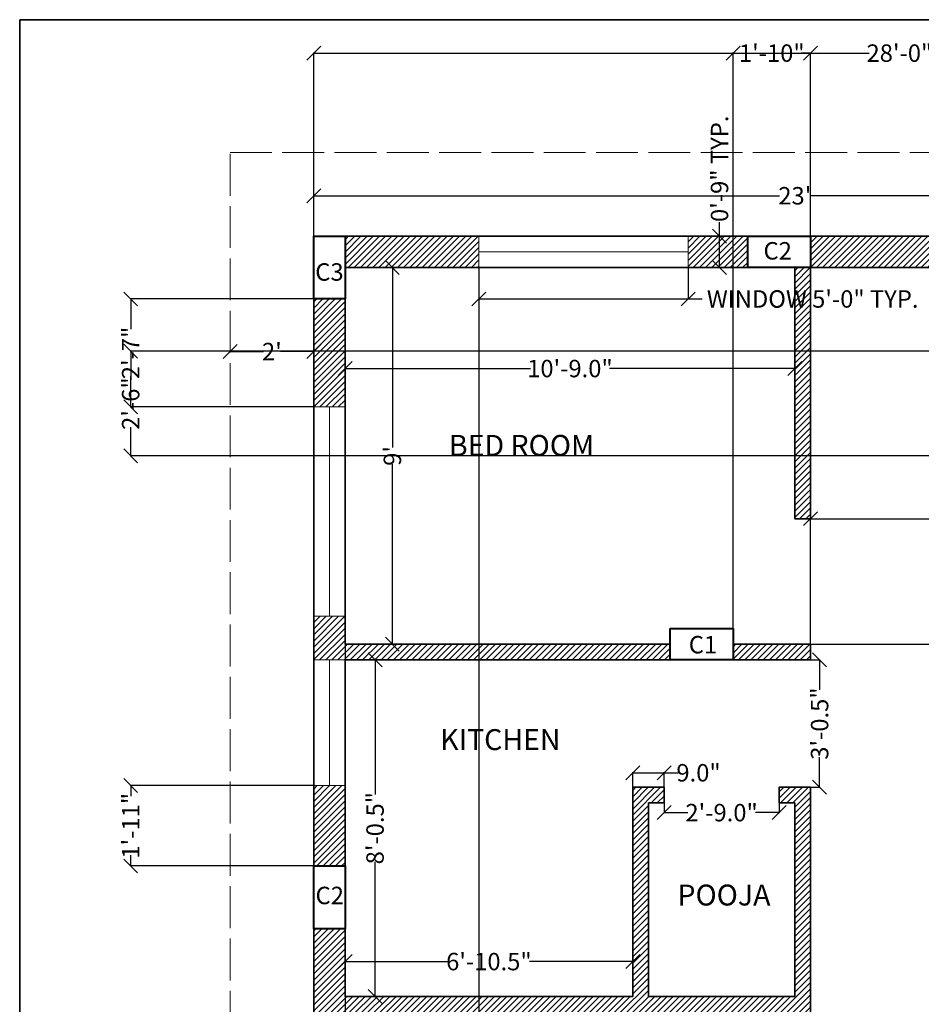
# Model space of a CAD drawing. Units: inches. Extents: x 72 to 538, y -43 to 598.
# Tile 3 of 4: x 72 to 331, y 316 to 598. Entities that reach past the tile are written whole.
import ezdxf

# ---------------------------------------------------------------- set-up
doc = ezdxf.new("R2010")
doc.units = ezdxf.units.IN
doc.header["$MEASUREMENT"] = 0
doc.linetypes.add('ACAD_ISO02W100', pattern=[15, 12, -3])
for name, color, linetype, lineweight in [('A-ANNO-DIMS', 2, 'Continuous', 18), ('A-ANNO-TEXT', 6, 'Continuous', 18), ('A-ANNO-TTLB', 7, 'Continuous', 35), ('A-AREA-IDEN', 7, 'Continuous', 25), ('A-COLS', 6, 'Continuous', 40), ('A-GLAZ', 4, 'Continuous', 18), ('A-WALL', 7, 'Continuous', 35), ('C-PROP', 3, 'ACAD_ISO02W100', 18)]:
    doc.layers.add(name, color=color, linetype=linetype, lineweight=lineweight)
doc.layers.add('A-WALL-PATT', color=30, linetype='Continuous', lineweight=13, true_color=0xf26722)
doc.styles.get("Standard").update_dxf_attribs({"font": 'arial.ttf'})
doc.dimstyles.get("Standard").update_dxf_attribs({"dimtxt": 5, "dimasz": 4, "dimexe": 0.18, "dimexo": 0.0625, "dimgap": 0.09, "dimtad": 0, "dimdec": 1, "dimzin": 0, "dimdsep": 46, "dimlunit": 3, "dimtxsty": 'Standard', "dimblk": 'OBLIQUE', "dimcen": 0.09, "dimadec": 0, "dimazin": 0, "dimtfac": 1, "dimtdec": 1, "dimtofl": 0, "dimtmove": 0, "dimatfit": 3, "dimfxl": 1, "dimtolj": 1, "dimtzin": 0, "dimarcsym": 0})

# ---------------------------------------------------------------- blocks, each defined once
blk = doc.blocks.new('_Oblique')
at = {"color": 0, "linetype": 'ByBlock', "lineweight": -2}
blk.add_line((-0.5, -0.5), (0.5, 0.5), dxfattribs=at)
blk = doc.blocks.new('*D2')
at = {"layer": 'A-ANNO-DIMS', "color": 0, "lineweight": -2, "transparency": 16777216}
for p, q in [((165.69, 527.12), (179.37, 527.12)), ((179.19, 527.12), (179.19, 475.51)), ((179.19, 419.12), (179.19, 470.73)), ((165.69, 419.12), (179.37, 419.12))]:
    blk.add_line(p, q, dxfattribs=at)
at = {"layer": 'Defpoints', "color": 0, "transparency": 16777216}
for p in [(165.63, 527.12), (165.63, 419.12), (179.19, 419.12)]:
    blk.add_point(p, dxfattribs=at)
at = {"layer": 'A-ANNO-DIMS', "color": 0, "lineweight": -2, "transparency": 16777216, "xscale": 4, "yscale": 4, "zscale": 4}
for p, rotation in [((179.19, 527.12), 90), ((179.19, 419.12), 270)]:
    blk.add_blockref('_Oblique', p, dxfattribs=dict(at, rotation=rotation))
at = {"layer": 'A-ANNO-DIMS', "color": 0, "transparency": 16777216, "insert": (179.19, 473.12), "char_height": 5, "attachment_point": 5, "rotation": 90}
blk.add_mtext("\\A1;9'", dxfattribs=at)
blk = doc.blocks.new('*D3')
at = {"layer": 'A-ANNO-DIMS', "color": 0, "lineweight": -2, "transparency": 16777216}
for p, q in [((165.63, 502.3), (165.63, 497.99)), ((294.63, 502.3), (294.63, 497.99)), ((165.63, 498.17), (218.77, 498.17)), ((294.63, 498.17), (241.48, 498.17))]:
    blk.add_line(p, q, dxfattribs=at)
at = {"layer": 'Defpoints', "color": 0, "transparency": 16777216}
for p in [(165.63, 502.36), (294.63, 502.36), (294.63, 498.17)]:
    blk.add_point(p, dxfattribs=at)
at = {"layer": 'A-ANNO-DIMS', "color": 0, "lineweight": -2, "transparency": 16777216, "xscale": 4, "yscale": 4, "zscale": 4, "rotation": 180}
blk.add_blockref('_Oblique', (165.63, 498.17), dxfattribs=at)
at = {"layer": 'A-ANNO-DIMS', "color": 0, "lineweight": -2, "transparency": 16777216, "xscale": 4, "yscale": 4, "zscale": 4}
blk.add_blockref('_Oblique', (294.63, 498.17), dxfattribs=at)
at = {"layer": 'A-ANNO-DIMS', "color": 0, "transparency": 16777216, "insert": (230.13, 498.17), "char_height": 5, "attachment_point": 5}
blk.add_mtext('\\A1;10\'-9.0"', dxfattribs=at)
blk = doc.blocks.new('*D6')
at = {"layer": 'A-ANNO-DIMS', "color": 0, "lineweight": -2, "transparency": 16777216}
for p, q in [((165.69, 414.62), (174.4, 414.62)), ((174.22, 414.62), (174.22, 376.02)), ((174.22, 318.12), (174.22, 356.72)), ((165.69, 318.12), (174.4, 318.12))]:
    blk.add_line(p, q, dxfattribs=at)
at = {"layer": 'Defpoints', "color": 0, "transparency": 16777216}
for p in [(165.63, 414.62), (174.22, 414.62), (165.63, 318.12)]:
    blk.add_point(p, dxfattribs=at)
at = {"layer": 'A-ANNO-DIMS', "color": 0, "lineweight": -2, "transparency": 16777216, "xscale": 4, "yscale": 4, "zscale": 4}
for p, rotation in [((174.22, 414.62), 90), ((174.22, 318.12), 270)]:
    blk.add_blockref('_Oblique', p, dxfattribs=dict(at, rotation=rotation))
at = {"layer": 'A-ANNO-DIMS', "color": 0, "transparency": 16777216, "insert": (174.22, 366.37), "char_height": 5, "attachment_point": 5, "rotation": 90}
blk.add_mtext('\\A1;8\'-0.5"', dxfattribs=at)
blk = doc.blocks.new('*D7')
at = {"layer": 'A-ANNO-DIMS', "color": 0, "lineweight": -2, "transparency": 16777216}
for p, q in [((165.63, 318.18), (165.63, 328.3)), ((165.63, 328.12), (195.28, 328.12)), ((248.13, 328.12), (218.48, 328.12)), ((248.13, 318.18), (248.13, 328.3))]:
    blk.add_line(p, q, dxfattribs=at)
at = {"layer": 'Defpoints', "color": 0, "transparency": 16777216}
for p in [(248.13, 328.12), (165.63, 318.12), (248.13, 318.12)]:
    blk.add_point(p, dxfattribs=at)
at = {"layer": 'A-ANNO-DIMS', "color": 0, "lineweight": -2, "transparency": 16777216, "xscale": 4, "yscale": 4, "zscale": 4, "rotation": 180}
blk.add_blockref('_Oblique', (165.63, 328.12), dxfattribs=at)
at = {"layer": 'A-ANNO-DIMS', "color": 0, "lineweight": -2, "transparency": 16777216, "xscale": 4, "yscale": 4, "zscale": 4}
blk.add_blockref('_Oblique', (248.13, 328.12), dxfattribs=at)
at = {"layer": 'A-ANNO-DIMS', "color": 0, "transparency": 16777216, "insert": (206.88, 328.12), "char_height": 5, "attachment_point": 5}
blk.add_mtext('\\A1;6\'-10.5"', dxfattribs=at)
blk = doc.blocks.new('*D8')
at = {"layer": 'A-ANNO-DIMS', "color": 0, "lineweight": -2, "transparency": 16777216}
for p, q in [((248.13, 378.18), (248.13, 382.44)), ((248.13, 382.26), (257.13, 382.26)), ((257.13, 378.18), (257.13, 382.44)), ((257.13, 382.26), (261.13, 382.26))]:
    blk.add_line(p, q, dxfattribs=at)
at = {"layer": 'Defpoints', "color": 0, "transparency": 16777216}
for p in [(257.13, 382.26), (248.13, 378.12), (257.13, 378.12)]:
    blk.add_point(p, dxfattribs=at)
at = {"layer": 'A-ANNO-DIMS', "color": 0, "lineweight": -2, "transparency": 16777216, "xscale": 4, "yscale": 4, "zscale": 4, "rotation": 180}
blk.add_blockref('_Oblique', (248.13, 382.26), dxfattribs=at)
at = {"layer": 'A-ANNO-DIMS', "color": 0, "lineweight": -2, "transparency": 16777216, "xscale": 4, "yscale": 4, "zscale": 4}
blk.add_blockref('_Oblique', (257.13, 382.26), dxfattribs=at)
at = {"layer": 'A-ANNO-DIMS', "color": 0, "transparency": 16777216, "insert": (267.01, 382.26), "char_height": 5, "attachment_point": 5}
blk.add_mtext('\\A1;9.0"', dxfattribs=at)
blk = doc.blocks.new('*D9')
at = {"layer": 'A-ANNO-DIMS', "color": 0, "lineweight": -2, "transparency": 16777216}
for p, q in [((257.13, 378.06), (257.13, 370.65)), ((290.13, 378.06), (290.13, 370.65)), ((257.13, 370.83), (263.94, 370.83)), ((290.13, 370.83), (283.32, 370.83))]:
    blk.add_line(p, q, dxfattribs=at)
at = {"layer": 'Defpoints', "color": 0, "transparency": 16777216}
for p in [(257.13, 378.12), (290.13, 378.12), (290.13, 370.83)]:
    blk.add_point(p, dxfattribs=at)
at = {"layer": 'A-ANNO-DIMS', "color": 0, "lineweight": -2, "transparency": 16777216, "xscale": 4, "yscale": 4, "zscale": 4, "rotation": 180}
blk.add_blockref('_Oblique', (257.13, 370.83), dxfattribs=at)
at = {"layer": 'A-ANNO-DIMS', "color": 0, "lineweight": -2, "transparency": 16777216, "xscale": 4, "yscale": 4, "zscale": 4}
blk.add_blockref('_Oblique', (290.13, 370.83), dxfattribs=at)
at = {"layer": 'A-ANNO-DIMS', "color": 0, "transparency": 16777216, "insert": (273.63, 370.83), "char_height": 5, "attachment_point": 5}
blk.add_mtext('\\A1;2\'-9.0"', dxfattribs=at)
blk = doc.blocks.new('*D10')
at = {"layer": 'A-ANNO-DIMS', "color": 0, "lineweight": -2, "transparency": 16777216}
for p, q in [((299.19, 414.62), (301.92, 414.62)), ((301.74, 414.62), (301.74, 406.02)), ((301.74, 378.12), (301.74, 386.72)), ((299.19, 378.12), (301.92, 378.12))]:
    blk.add_line(p, q, dxfattribs=at)
at = {"layer": 'Defpoints', "color": 0, "transparency": 16777216}
for p in [(299.13, 414.62), (299.13, 378.12), (301.74, 378.12)]:
    blk.add_point(p, dxfattribs=at)
at = {"layer": 'A-ANNO-DIMS', "color": 0, "lineweight": -2, "transparency": 16777216, "xscale": 4, "yscale": 4, "zscale": 4}
for p, rotation in [((301.74, 414.62), 90), ((301.74, 378.12), 270)]:
    blk.add_blockref('_Oblique', p, dxfattribs=dict(at, rotation=rotation))
at = {"layer": 'A-ANNO-DIMS', "color": 0, "transparency": 16777216, "insert": (301.74, 396.37), "char_height": 5, "attachment_point": 5, "rotation": 90}
blk.add_mtext('\\A1;3\'-0.5"', dxfattribs=at)
blk = doc.blocks.new('*D26')
at = {"layer": 'A-ANNO-DIMS', "color": 0, "lineweight": -2, "transparency": 16777216}
for p, q in [((299.13, 455.18), (299.13, 455.3)), ((299.13, 455.12), (350.02, 455.12)), ((423.63, 455.12), (372.73, 455.12)), ((423.63, 455.18), (423.63, 455.3))]:
    blk.add_line(p, q, dxfattribs=at)
at = {"layer": 'Defpoints', "color": 0, "transparency": 16777216}
for p in [(299.13, 455.12), (423.63, 455.12), (423.63, 455.12)]:
    blk.add_point(p, dxfattribs=at)
at = {"layer": 'A-ANNO-DIMS', "color": 0, "lineweight": -2, "transparency": 16777216, "xscale": 4, "yscale": 4, "zscale": 4, "rotation": 180}
blk.add_blockref('_Oblique', (299.13, 455.12), dxfattribs=at)
at = {"layer": 'A-ANNO-DIMS', "color": 0, "lineweight": -2, "transparency": 16777216, "xscale": 4, "yscale": 4, "zscale": 4}
blk.add_blockref('_Oblique', (423.63, 455.12), dxfattribs=at)
at = {"layer": 'A-ANNO-DIMS', "color": 0, "transparency": 16777216, "insert": (361.38, 455.12), "char_height": 5, "attachment_point": 5}
blk.add_mtext('\\A1;10\'-4.5"', dxfattribs=at)
blk = doc.blocks.new('*D37')
at = {"layer": 'A-ANNO-DIMS', "color": 0, "lineweight": -2, "transparency": 16777216}
for p, q in [((156.63, 536.18), (156.63, 547.9)), ((432.63, 536.18), (432.63, 547.9)), ((156.63, 547.72), (290.25, 547.72)), ((432.63, 547.72), (299, 547.72))]:
    blk.add_line(p, q, dxfattribs=at)
at = {"layer": 'Defpoints', "color": 0, "transparency": 16777216}
for p in [(432.63, 547.72), (156.63, 536.12), (432.63, 536.12)]:
    blk.add_point(p, dxfattribs=at)
at = {"layer": 'A-ANNO-DIMS', "color": 0, "lineweight": -2, "transparency": 16777216, "xscale": 4, "yscale": 4, "zscale": 4, "rotation": 180}
blk.add_blockref('_Oblique', (156.63, 547.72), dxfattribs=at)
at = {"layer": 'A-ANNO-DIMS', "color": 0, "lineweight": -2, "transparency": 16777216, "xscale": 4, "yscale": 4, "zscale": 4}
blk.add_blockref('_Oblique', (432.63, 547.72), dxfattribs=at)
at = {"layer": 'A-ANNO-DIMS', "color": 0, "transparency": 16777216, "insert": (294.63, 547.72), "char_height": 5, "attachment_point": 5}
blk.add_mtext("\\A1;23'", dxfattribs=at)
blk = doc.blocks.new('*D39')
at = {"layer": 'A-ANNO-DIMS', "color": 0, "lineweight": -2, "transparency": 16777216}
for p, q in [((132.63, 503.09), (132.63, 503.21)), ((132.63, 503.03), (142.2, 503.03)), ((156.63, 503.03), (147.06, 503.03)), ((156.63, 503.09), (156.63, 503.21))]:
    blk.add_line(p, q, dxfattribs=at)
at = {"layer": 'Defpoints', "color": 0, "transparency": 16777216}
for p in [(132.63, 503.03), (156.63, 503.03), (156.63, 503.03)]:
    blk.add_point(p, dxfattribs=at)
at = {"layer": 'A-ANNO-DIMS', "color": 0, "lineweight": -2, "transparency": 16777216, "xscale": 4, "yscale": 4, "zscale": 4, "rotation": 180}
blk.add_blockref('_Oblique', (132.63, 503.03), dxfattribs=at)
at = {"layer": 'A-ANNO-DIMS', "color": 0, "lineweight": -2, "transparency": 16777216, "xscale": 4, "yscale": 4, "zscale": 4}
blk.add_blockref('_Oblique', (156.63, 503.03), dxfattribs=at)
at = {"layer": 'A-ANNO-DIMS', "color": 0, "transparency": 16777216, "insert": (144.63, 503.03), "char_height": 5, "attachment_point": 5}
blk.add_mtext("\\A1;2'", dxfattribs=at)
blk = doc.blocks.new('COL-9X18')
for p, q in [((0, 18), (9, 18)), ((0, 0), (0, 18)), ((9, 18), (9, 0)), ((9, 0), (0, 0))]:
    blk.add_line(p, q)
blk = doc.blocks.new('WIN-60')
for p, q in [((0, 9), (0, 0)), ((60, 9), (60, 0)), ((0, 4.5), (60, 4.5))]:
    blk.add_line(p, q)
blk = doc.blocks.new('WIN-36')
for p, q in [((9, 36), (0, 36)), ((4.5, 36), (4.5, 0)), ((9, 0), (0, 0))]:
    blk.add_line(p, q)
blk = doc.blocks.new('*D46')
at = {"layer": 'A-ANNO-DIMS', "color": 0, "lineweight": -2, "transparency": 16777216}
for p, q in [((204.03, 527.06), (204.03, 517.94)), ((264.03, 527.06), (264.03, 517.94)), ((204.03, 518.12), (264.03, 518.12)), ((264.03, 518.12), (268.03, 518.12))]:
    blk.add_line(p, q, dxfattribs=at)
at = {"layer": 'Defpoints', "color": 0, "transparency": 16777216}
for p in [(204.03, 527.12), (264.03, 527.12), (264.03, 518.12)]:
    blk.add_point(p, dxfattribs=at)
at = {"layer": 'A-ANNO-DIMS', "color": 0, "lineweight": -2, "transparency": 16777216, "xscale": 4, "yscale": 4, "zscale": 4, "rotation": 180}
blk.add_blockref('_Oblique', (204.03, 518.12), dxfattribs=at)
at = {"layer": 'A-ANNO-DIMS', "color": 0, "lineweight": -2, "transparency": 16777216, "xscale": 4, "yscale": 4, "zscale": 4}
blk.add_blockref('_Oblique', (264.03, 518.12), dxfattribs=at)
at = {"layer": 'A-ANNO-DIMS', "color": 0, "transparency": 16777216, "insert": (299.76, 518.12), "char_height": 5, "attachment_point": 5}
blk.add_mtext('\\A1;WINDOW 5\'-0" TYP.', dxfattribs=at)
blk = doc.blocks.new('*D47')
at = {"layer": 'A-ANNO-DIMS', "color": 0, "lineweight": -2, "transparency": 16777216}
for p, q in [((273.03, 536.12), (273.03, 540.12)), ((264.1, 536.12), (273.21, 536.12)), ((273.03, 527.12), (273.03, 536.12)), ((264.1, 527.12), (273.21, 527.12))]:
    blk.add_line(p, q, dxfattribs=at)
at = {"layer": 'Defpoints', "color": 0, "transparency": 16777216}
for p in [(264.03, 536.12), (273.03, 536.12), (264.03, 527.12)]:
    blk.add_point(p, dxfattribs=at)
at = {"layer": 'A-ANNO-DIMS', "color": 0, "lineweight": -2, "transparency": 16777216, "xscale": 4, "yscale": 4, "zscale": 4}
for p, rotation in [((273.03, 536.12), 90), ((273.03, 527.12), 270)]:
    blk.add_blockref('_Oblique', p, dxfattribs=dict(at, rotation=rotation))
at = {"layer": 'A-ANNO-DIMS', "color": 0, "transparency": 16777216, "insert": (273.03, 555.45), "char_height": 5, "attachment_point": 5, "rotation": 90}
blk.add_mtext('\\A1;0\'-9" TYP.', dxfattribs=at)
blk = doc.blocks.new('*D52')
at = {"layer": 'A-ANNO-DIMS', "color": 0, "lineweight": -2, "transparency": 16777216}
for p, q in [((156.63, 536.18), (156.63, 588.8)), ((156.63, 588.62), (315.91, 588.62)), ((492.63, 588.62), (333.35, 588.62)), ((492.63, 536.18), (492.63, 588.8))]:
    blk.add_line(p, q, dxfattribs=at)
at = {"layer": 'Defpoints', "color": 0, "transparency": 16777216}
for p in [(492.63, 588.62), (156.63, 536.12), (492.63, 536.12)]:
    blk.add_point(p, dxfattribs=at)
at = {"layer": 'A-ANNO-DIMS', "color": 0, "lineweight": -2, "transparency": 16777216, "xscale": 4, "yscale": 4, "zscale": 4, "rotation": 180}
blk.add_blockref('_Oblique', (156.63, 588.62), dxfattribs=at)
at = {"layer": 'A-ANNO-DIMS', "color": 0, "lineweight": -2, "transparency": 16777216, "xscale": 4, "yscale": 4, "zscale": 4}
blk.add_blockref('_Oblique', (492.63, 588.62), dxfattribs=at)
at = {"layer": 'A-ANNO-DIMS', "color": 0, "transparency": 16777216, "insert": (324.63, 588.62), "char_height": 5, "attachment_point": 5}
blk.add_mtext('\\A1;28\'-0"', dxfattribs=at)
blk = doc.blocks.new('*D57')
at = {"layer": 'A-ANNO-DIMS', "color": 0, "lineweight": -2, "transparency": 16777216}
for p, q in [((165.63, 527.06), (165.63, -35.94)), ((204.03, 527.06), (204.03, -35.94)), ((165.63, -35.76), (172.27, -35.76)), ((204.03, -35.76), (197.39, -35.76))]:
    blk.add_line(p, q, dxfattribs=at)
at = {"layer": 'Defpoints', "color": 0, "transparency": 16777216}
for p in [(165.63, 527.12), (204.03, 527.12), (204.03, -35.76)]:
    blk.add_point(p, dxfattribs=at)
at = {"layer": 'A-ANNO-DIMS', "color": 0, "lineweight": -2, "transparency": 16777216, "xscale": 4, "yscale": 4, "zscale": 4, "rotation": 180}
blk.add_blockref('_Oblique', (165.63, -35.76), dxfattribs=at)
at = {"layer": 'A-ANNO-DIMS', "color": 0, "lineweight": -2, "transparency": 16777216, "xscale": 4, "yscale": 4, "zscale": 4}
blk.add_blockref('_Oblique', (204.03, -35.76), dxfattribs=at)
at = {"layer": 'A-ANNO-DIMS', "color": 0, "transparency": 16777216, "insert": (184.83, -35.76), "char_height": 5, "attachment_point": 5}
blk.add_mtext('\\A1;3\'-2 1/2"', dxfattribs=at)
blk = doc.blocks.new('*D58')
at = {"layer": 'A-ANNO-DIMS', "color": 0, "lineweight": -2, "transparency": 16777216}
for p, q in [((156.57, 518.12), (103.95, 518.12)), ((104.13, 518.12), (104.13, 509.43)), ((104.13, 487.18), (104.13, 495.87)), ((156.57, 487.18), (103.95, 487.18))]:
    blk.add_line(p, q, dxfattribs=at)
at = {"layer": 'Defpoints', "color": 0, "transparency": 16777216}
for p in [(156.63, 518.12), (104.13, 487.18), (156.63, 487.18)]:
    blk.add_point(p, dxfattribs=at)
at = {"layer": 'A-ANNO-DIMS', "color": 0, "lineweight": -2, "transparency": 16777216, "xscale": 4, "yscale": 4, "zscale": 4}
for p, rotation in [((104.13, 518.12), 90), ((104.13, 487.18), 270)]:
    blk.add_blockref('_Oblique', p, dxfattribs=dict(at, rotation=rotation))
at = {"layer": 'A-ANNO-DIMS', "color": 0, "transparency": 16777216, "insert": (104.13, 502.65), "char_height": 5, "attachment_point": 5, "rotation": 90}
blk.add_mtext('\\A1;2\'-7"', dxfattribs=at)
blk = doc.blocks.new('*D62')
at = {"layer": 'A-ANNO-DIMS', "color": 0, "lineweight": -2, "transparency": 16777216}
for p, q in [((339.57, 503.12), (103.95, 503.12)), ((104.13, 503.12), (104.13, 494.9)), ((104.13, 473.12), (104.13, 481.34)), ((339.57, 473.12), (103.95, 473.12))]:
    blk.add_line(p, q, dxfattribs=at)
at = {"layer": 'Defpoints', "color": 0, "transparency": 16777216}
for p in [(339.63, 503.12), (104.13, 473.12), (339.63, 473.12)]:
    blk.add_point(p, dxfattribs=at)
at = {"layer": 'A-ANNO-DIMS', "color": 0, "lineweight": -2, "transparency": 16777216, "xscale": 4, "yscale": 4, "zscale": 4}
for p, rotation in [((104.13, 503.12), 90), ((104.13, 473.12), 270)]:
    blk.add_blockref('_Oblique', p, dxfattribs=dict(at, rotation=rotation))
at = {"layer": 'A-ANNO-DIMS', "color": 0, "transparency": 16777216, "insert": (104.13, 488.12), "char_height": 5, "attachment_point": 5, "rotation": 90}
blk.add_mtext('\\A1;2\'-6"', dxfattribs=at)
blk = doc.blocks.new('*D63')
at = {"layer": 'A-ANNO-DIMS', "color": 0, "lineweight": -2, "transparency": 16777216}
for p, q in [((294.69, 455.12), (521.31, 455.12)), ((521.13, 455.12), (521.13, 443.85)), ((521.13, 419.12), (521.13, 430.39)), ((299.19, 419.12), (521.31, 419.12))]:
    blk.add_line(p, q, dxfattribs=at)
at = {"layer": 'Defpoints', "color": 0, "transparency": 16777216}
for p in [(294.63, 455.12), (299.13, 419.12), (521.13, 419.12)]:
    blk.add_point(p, dxfattribs=at)
at = {"layer": 'A-ANNO-DIMS', "color": 0, "lineweight": -2, "transparency": 16777216, "xscale": 4, "yscale": 4, "zscale": 4}
for p, rotation in [((521.13, 455.12), 90), ((521.13, 419.12), 270)]:
    blk.add_blockref('_Oblique', p, dxfattribs=dict(at, rotation=rotation))
at = {"layer": 'A-ANNO-DIMS', "color": 0, "transparency": 16777216, "insert": (521.13, 437.12), "char_height": 5, "attachment_point": 5, "rotation": 90}
blk.add_mtext('\\A1;3\'-0"', dxfattribs=at)
blk = doc.blocks.new('*D68')
at = {"layer": 'A-ANNO-DIMS', "color": 0, "lineweight": -2, "transparency": 16777216}
for p, q in [((156.57, 378.62), (103.95, 378.62)), ((104.13, 378.62), (104.13, 375.52)), ((104.13, 355.53), (104.13, 358.63)), ((156.57, 355.53), (103.95, 355.53))]:
    blk.add_line(p, q, dxfattribs=at)
at = {"layer": 'Defpoints', "color": 0, "transparency": 16777216}
for p in [(104.13, 378.62), (156.63, 378.62), (156.63, 355.53)]:
    blk.add_point(p, dxfattribs=at)
at = {"layer": 'A-ANNO-DIMS', "color": 0, "lineweight": -2, "transparency": 16777216, "xscale": 4, "yscale": 4, "zscale": 4}
for p, rotation in [((104.13, 378.62), 90), ((104.13, 355.53), 270)]:
    blk.add_blockref('_Oblique', p, dxfattribs=dict(at, rotation=rotation))
at = {"layer": 'A-ANNO-DIMS', "color": 0, "transparency": 16777216, "insert": (104.13, 367.07), "char_height": 5, "attachment_point": 5, "rotation": 90}
blk.add_mtext('\\A1;1\'-11"', dxfattribs=at)
blk = doc.blocks.new('*D70')
at = {"layer": 'A-ANNO-DIMS', "color": 0, "lineweight": -2, "transparency": 16777216}
for p, q in [((276.91, 419.18), (276.91, 588.8)), ((276.91, 588.62), (279.58, 588.62)), ((299.13, 588.62), (296.46, 588.62)), ((299.13, 419.18), (299.13, 588.8))]:
    blk.add_line(p, q, dxfattribs=at)
at = {"layer": 'Defpoints', "color": 0, "transparency": 16777216}
for p in [(299.13, 588.62), (276.91, 419.12), (299.13, 419.12)]:
    blk.add_point(p, dxfattribs=at)
at = {"layer": 'A-ANNO-DIMS', "color": 0, "lineweight": -2, "transparency": 16777216, "xscale": 4, "yscale": 4, "zscale": 4, "rotation": 180}
blk.add_blockref('_Oblique', (276.91, 588.62), dxfattribs=at)
at = {"layer": 'A-ANNO-DIMS', "color": 0, "lineweight": -2, "transparency": 16777216, "xscale": 4, "yscale": 4, "zscale": 4}
blk.add_blockref('_Oblique', (299.13, 588.62), dxfattribs=at)
at = {"layer": 'A-ANNO-DIMS', "color": 0, "transparency": 16777216, "insert": (288.02, 588.62), "char_height": 5, "attachment_point": 5}
blk.add_mtext('\\A1;1\'-10"', dxfattribs=at)

msp = doc.modelspace()

# ---------------------------------------------------------------- hatches: boundary and pattern name
at = {"layer": 'A-WALL-PATT'}
h = msp.add_hatch(dxfattribs=at)
h.set_pattern_fill('ANSI31', color=256, scale=10)
h.paths.add_polyline_path([(204.03, 536.12), (165.63, 536.12), (165.63, 527.12), (204.03, 527.12)])
h.paths.add_polyline_path([(165.63, 487.18), (165.63, 518.12), (156.63, 518.12), (156.63, 487.18)])
h.paths.add_polyline_path([(374.85, 253.74), (416.04, 253.74), (416.04, 266.11), (374.85, 266.11)], flags=9)
h.paths.add_polyline_path([(358.05, 165.41), (382.02, 165.41), (382.02, 177.78), (358.05, 177.78)], flags=9)
h.paths.add_polyline_path([(258.82, 340.82), (290.25, 340.82), (290.25, 353.18), (258.82, 353.18)], flags=9)
h.paths.add_polyline_path([(190.8, 385.39), (230.59, 385.39), (230.59, 397.75), (190.8, 397.75)], flags=9)
h.paths.add_polyline_path([(259.76, 122.35), (291.18, 122.35), (291.18, 134.72), (259.76, 134.72)], flags=9)
h.paths.add_polyline_path([(192.66, 147.9), (232.45, 147.9), (232.45, 160.26), (192.66, 160.26)], flags=9)
h.paths.add_polyline_path([(197.84, 250.21), (246.48, 250.21), (246.48, 262.58), (197.84, 262.58)], flags=9)
h.paths.add_polyline_path([(329.22, 365.75), (353.18, 365.75), (353.18, 378.11), (329.22, 378.11)], flags=9)
h.paths.add_polyline_path([(351.21, 489.41), (392.39, 489.41), (392.39, 501.77), (351.21, 501.77)], flags=9)
h.paths.add_polyline_path([(193.31, 469.76), (241.95, 469.76), (241.95, 482.12), (193.31, 482.12)], flags=9)
h.paths.add_polyline_path([(262.62, 413.67), (274.04, 413.67), (274.04, 423.97), (262.62, 423.97)], flags=9)
h.paths.add_polyline_path([(155.57, 341.76), (167, 341.76), (167, 352.06), (155.57, 352.06)], flags=9)
h.paths.add_polyline_path([(155.43, 129.83), (166.86, 129.83), (166.86, 140.14), (155.43, 140.14)], flags=9)
h.paths.add_polyline_path([(293.27, 137.19), (304.7, 137.19), (304.7, 147.49), (293.27, 147.49)], flags=9)
h.paths.add_polyline_path([(440.6, 145.74), (452.03, 145.74), (452.03, 156.04), (440.6, 156.04)], flags=9)
h.paths.add_polyline_path([(422.43, 340.03), (433.86, 340.03), (433.86, 350.33), (422.43, 350.33)], flags=9)
h.paths.add_polyline_path([(155.47, 520.54), (166.9, 520.54), (166.9, 530.84), (155.47, 530.84)], flags=9)
h.paths.add_polyline_path([(348.1, 449.93), (374.22, 449.93), (374.22, 460.24), (348.1, 460.24)], flags=9)
h.paths.add_polyline_path([(417.29, 368.09), (417.29, 394.21), (406.99, 394.21), (406.99, 368.09)], flags=9)
h.paths.add_polyline_path([(422.51, 520.96), (433.94, 520.96), (433.94, 531.26), (422.51, 531.26)], flags=9)
h.paths.add_polyline_path([(284.05, 526.61), (295.48, 526.61), (295.48, 536.92), (284.05, 536.92)], flags=9)
h = msp.add_hatch(dxfattribs=at)
h.set_pattern_fill('ANSI31', color=256, scale=10)
h.paths.add_polyline_path([(432.63, 468.62), (432.63, 518.12), (423.63, 518.12), (423.63, 473.12), (339.63, 473.12), (335.13, 473.12), (335.13, 468.62), (423.63, 468.62), (423.63, 354.62), (432.63, 354.62)])
h.paths.add_polyline_path([(450.63, 231.12), (450.63, 240.93), (441.63, 240.93), (441.63, 235.62), (357.63, 235.62), (353.13, 235.62), (353.13, 231.12), (441.63, 231.12)])
h.paths.add_polyline_path([(374.85, 253.74), (416.04, 253.74), (416.04, 266.11), (374.85, 266.11)], flags=9)
h.paths.add_polyline_path([(358.05, 165.41), (382.02, 165.41), (382.02, 177.78), (358.05, 177.78)], flags=9)
h.paths.add_polyline_path([(258.82, 340.82), (290.25, 340.82), (290.25, 353.18), (258.82, 353.18)], flags=9)
h.paths.add_polyline_path([(190.8, 385.39), (230.59, 385.39), (230.59, 397.75), (190.8, 397.75)], flags=9)
h.paths.add_polyline_path([(259.76, 122.35), (291.18, 122.35), (291.18, 134.72), (259.76, 134.72)], flags=9)
h.paths.add_polyline_path([(192.66, 147.9), (232.45, 147.9), (232.45, 160.26), (192.66, 160.26)], flags=9)
h.paths.add_polyline_path([(197.84, 250.21), (246.48, 250.21), (246.48, 262.58), (197.84, 262.58)], flags=9)
h.paths.add_polyline_path([(329.22, 365.75), (353.18, 365.75), (353.18, 378.11), (329.22, 378.11)], flags=9)
h.paths.add_polyline_path([(351.21, 489.41), (392.39, 489.41), (392.39, 501.77), (351.21, 501.77)], flags=25)
h.paths.add_polyline_path([(193.31, 469.76), (241.95, 469.76), (241.95, 482.12), (193.31, 482.12)], flags=9)
h.paths.add_polyline_path([(262.62, 413.67), (274.04, 413.67), (274.04, 423.97), (262.62, 423.97)], flags=9)
h.paths.add_polyline_path([(155.57, 341.76), (167, 341.76), (167, 352.06), (155.57, 352.06)], flags=9)
h.paths.add_polyline_path([(155.43, 129.83), (166.86, 129.83), (166.86, 140.14), (155.43, 140.14)], flags=9)
h.paths.add_polyline_path([(293.27, 137.19), (304.7, 137.19), (304.7, 147.49), (293.27, 147.49)], flags=9)
h.paths.add_polyline_path([(440.6, 145.74), (452.03, 145.74), (452.03, 156.04), (440.6, 156.04)], flags=9)
h.paths.add_polyline_path([(422.43, 340.03), (433.86, 340.03), (433.86, 350.33), (422.43, 350.33)], flags=9)
h.paths.add_polyline_path([(422.51, 520.96), (433.94, 520.96), (433.94, 531.26), (422.51, 531.26)], flags=9)
h.paths.add_polyline_path([(284.05, 526.61), (295.48, 526.61), (295.48, 536.92), (284.05, 536.92)], flags=9)
h.paths.add_polyline_path([(155.47, 520.54), (166.9, 520.54), (166.9, 530.84), (155.47, 530.84)], flags=9)
h = msp.add_hatch(dxfattribs=at)
h.set_pattern_fill('ANSI31', color=256, scale=10)
h.paths.add_polyline_path([(165.63, 427.18), (156.63, 427.18), (156.63, 414.62), (165.63, 414.62), (258.91, 414.62), (258.91, 419.12), (165.63, 419.12)])
h.paths.add_polyline_path([(165.63, 378.62), (156.63, 378.62), (156.63, 355.53), (165.63, 355.53)])
h.paths.add_polyline_path([(299.13, 378.12), (290.13, 378.12), (290.13, 373.62), (294.63, 373.62), (294.63, 318.12), (252.63, 318.12), (252.63, 373.62), (257.13, 373.62), (257.13, 378.12), (248.13, 378.12), (248.13, 318.12), (165.63, 318.12), (165.63, 337.53), (156.63, 337.53), (156.63, 294.2), (165.63, 294.2), (165.63, 313.62), (294.63, 313.62), (294.63, 289.62), (312.63, 289.62), (312.63, 235.62), (294.63, 235.62), (294.63, 231.12), (317.13, 231.12), (317.13, 289.62), (353.13, 289.62), (353.13, 265.62), (357.63, 265.62), (357.63, 289.62), (441.63, 289.62), (441.63, 264.93), (450.63, 264.93), (450.63, 294.12), (432.63, 294.12), (299.13, 294.12)])
h.paths.add_polyline_path([(299.13, 195.12), (165.63, 195.12), (165.63, 234.2), (156.63, 234.2), (156.63, 144.66), (165.63, 144.66), (165.63, 190.62), (299.13, 190.62)])
h.paths.add_polyline_path([(165.63, 126.66), (156.63, 126.66), (156.63, 80.12), (212.13, 80.12), (212.13, 89.12), (165.63, 89.12)])
h.paths.add_polyline_path([(310.61, 89.12), (299.13, 89.12), (299.13, 137.87), (294.63, 137.87), (294.63, 89.12), (252.63, 89.12), (252.63, 144.62), (257.13, 144.62), (257.13, 149.12), (248.13, 149.12), (248.13, 89.12), (248.13, 80.12), (310.61, 80.12)])
h.paths.add_polyline_path([(450.63, 142.12), (441.63, 142.12), (441.63, 89.12), (433.82, 89.12), (433.82, 80.12), (450.63, 80.12)])
h.paths.add_polyline_path([(450.63, 171.12), (446.13, 171.12), (441.63, 171.12), (441.63, 160.12), (450.63, 160.12)])
h.paths.add_polyline_path([(281.13, 536.12), (264.03, 536.12), (264.03, 527.12), (281.13, 527.12)])
h.paths.add_polyline_path([(339.63, 536.12), (299.13, 536.12), (299.13, 527.12), (335.13, 527.12), (335.13, 503.12), (339.63, 503.12), (339.63, 527.12)])
h.paths.add_polyline_path([(299.13, 527.12), (294.63, 527.12), (294.63, 455.12), (299.13, 455.12)])
h.paths.add_polyline_path([(492.63, 536.12), (432.63, 536.12), (432.63, 527.12), (492.63, 527.12)])
h.paths.add_polyline_path([(423.63, 536.12), (363.63, 536.12), (363.63, 527.12), (423.63, 527.12)])
h.paths.add_polyline_path([(299.13, 419.12), (276.91, 419.12), (276.91, 414.62), (299.13, 414.62)])

# ---------------------------------------------------------------- linework, layer by layer
at = {"layer": 'A-ANNO-TTLB'}
msp.add_lwpolyline([(72.29, 598.2), (537.75, 598.2), (537.75, -7.26), (72.29, -7.26)], close=True, dxfattribs=at)
at = {"layer": 'A-WALL'}
for p, q in [((156.63, 536.12), (432.63, 536.12)), ((156.63, 80.12), (156.63, 536.12)), ((165.63, 527.12), (294.63, 527.12)), ((165.63, 419.12), (165.63, 527.12)), ((294.63, 455.12), (294.63, 527.12)), ((299.13, 527.12), (335.13, 527.12)), ((299.13, 455.12), (299.13, 527.12)), ((294.63, 455.12), (299.13, 455.12)), ((165.63, 419.12), (258.91, 419.12)), ((276.91, 419.12), (299.13, 419.12)), ((299.13, 414.62), (299.13, 419.12)), ((165.63, 414.62), (299.13, 414.62)), ((165.63, 318.12), (165.63, 414.62)), ((248.13, 318.12), (248.13, 378.12)), ((248.13, 378.12), (257.13, 378.12)), ((248.13, 378.12), (257.13, 378.12)), ((257.13, 378.12), (257.13, 373.62)), ((290.13, 378.12), (290.13, 373.62)), ((290.13, 378.12), (299.13, 378.12)), ((299.13, 294.12), (299.13, 378.12)), ((252.63, 318.12), (252.63, 373.62)), ((252.63, 373.62), (257.13, 373.62)), ((290.13, 373.62), (294.63, 373.62)), ((294.63, 318.12), (294.63, 373.62)), ((165.63, 318.12), (248.13, 318.12)), ((252.63, 318.12), (294.63, 318.12))]:
    msp.add_line(p, q, dxfattribs=at)
at = {"layer": 'C-PROP'}
for p, q in [((132.63, -7.26), (132.63, 560.12)), ((132.63, 560.12), (492.63, 560.12))]:
    msp.add_line(p, q, dxfattribs=at)

# ---------------------------------------------------------------- block references
at = {"layer": 'A-COLS'}
for p in [(156.63, 518.12), (156.63, 337.53)]:
    msp.add_blockref('COL-9X18', p, dxfattribs=at)
for p, rotation in [((299.13, 527.12), 89.99999999999969), ((276.91, 414.62), 90.00000000000043)]:
    msp.add_blockref('COL-9X18', p, dxfattribs=dict(at, rotation=rotation))
at = {"layer": 'A-GLAZ'}
for name, p in [('WIN-60', (204.03, 527.12)), ('WIN-36', (156.63, 378.62))]:
    msp.add_blockref(name, p, dxfattribs=at)
at = {"layer": 'A-GLAZ', "rotation": 269.9999999999998}
msp.add_blockref('WIN-60', (156.63, 487.18), dxfattribs=at)

# ---------------------------------------------------------------- texts
at = {"layer": 'A-ANNO-TEXT', "char_height": 5, "attachment_point": 1}
for s, insert in [('C2', (285.65, 534.43)), ('C3', (157.07, 528.36)), ('C1', (264.21, 421.49)), ('C2', (157.16, 349.58))]:
    msp.add_mtext_dynamic_manual_height_columns(s, width=12, gutter_width=1, heights=[0], dxfattribs=dict(at, insert=insert))
at = {"layer": 'A-AREA-IDEN', "char_height": 6, "attachment_point": 1}
for s, insert in [('BED ROOM', (195.42, 479.14)), ('KITCHEN', (192.92, 394.77)), ('POOJA', (260.97, 350.2))]:
    msp.add_mtext_dynamic_manual_height_columns(s, width=78.4308, gutter_width=1, heights=[0], dxfattribs=dict(at, insert=insert))

# ---------------------------------------------------------------- dimensions: what is measured, and where the dimension line sits
at = {"layer": 'A-ANNO-DIMS'}
for base, p1, p2, override, picture, middle in [((492.63, 588.62), (156.63, 536.12), (492.63, 536.12), {"dimdec": 1, "dimlfac": 1, "dimrnd": 0, "dimzin": 1, "dimdsep": 46, "dimlunit": 4, "dimfrac": 2}, '*D52', (324.63, 588.62)), ((299.13, 588.62), (276.91, 419.12), (299.13, 419.12), {"dimdec": 1, "dimlfac": 1, "dimrnd": 0, "dimzin": 1, "dimdsep": 46, "dimlunit": 4, "dimfrac": 2}, '*D70', (288.02, 588.62)), ((432.63, 547.72), (156.63, 536.12), (432.63, 536.12), {"dimclrd": 0, "dimclre": 0, "dimclrt": 0}, '*D37', (294.63, 547.72)), ((204.03, -35.76), (165.63, 527.12), (204.03, 527.12), {"dimdec": 1, "dimlfac": 1, "dimrnd": 0, "dimzin": 1, "dimdsep": 46, "dimlunit": 4, "dimfrac": 2}, '*D57', (184.83, -35.76)), ((156.63, 503.03), (132.63, 503.03), (156.63, 503.03), {"dimclrd": 0, "dimclre": 0, "dimclrt": 0}, '*D39', (144.63, 503.03)), ((294.63, 498.17), (165.63, 502.36), (294.63, 502.36), {"dimclrd": 0, "dimclre": 0, "dimclrt": 0}, '*D3', (230.13, 498.17)), ((423.63, 455.12), (299.13, 455.12), (423.63, 455.12), {"dimclrd": 0, "dimclre": 0, "dimclrt": 0}, '*D26', (361.38, 455.12)), ((257.13, 382.26), (248.13, 378.12), (257.13, 378.12), {"dimclrd": 0, "dimclre": 0, "dimclrt": 0}, '*D8', (267.01, 382.26)), ((290.13, 370.83), (257.13, 378.12), (290.13, 378.12), {"dimclrd": 0, "dimclre": 0, "dimclrt": 0}, '*D9', (273.63, 370.83)), ((248.13, 328.12), (165.63, 318.12), (248.13, 318.12), {"dimclrd": 0, "dimclre": 0, "dimclrt": 0}, '*D7', (206.88, 328.12))]:
    dim = msp.add_linear_dim(base=base, p1=p1, p2=p2, dimstyle='Standard', override=override, dxfattribs=at)
    dim.commit()
    dim.dimension.update_dxf_attribs({"geometry": picture, "text_midpoint": middle})
dim = msp.add_linear_dim(base=(273.03, 536.12), p1=(264.03, 527.12), p2=(264.03, 536.12), angle=90, text='<> TYP.', dimstyle='Standard', override={"dimdec": 1, "dimlfac": 1, "dimrnd": 0, "dimzin": 1, "dimdsep": 46, "dimlunit": 4, "dimfrac": 2}, dxfattribs=at)
dim.commit()
dim.dimension.update_dxf_attribs({"geometry": '*D47', "text_midpoint": (273.03, 555.45)})
for base, p1, p2, override, picture, middle in [((179.19, 419.12), (165.63, 527.12), (165.63, 419.12), {"dimclrd": 0, "dimclre": 0, "dimclrt": 0}, '*D2', (179.19, 473.12)), ((104.13, 487.18), (156.63, 518.12), (156.63, 487.18), {"dimdec": 1, "dimlfac": 1, "dimrnd": 0, "dimzin": 1, "dimdsep": 46, "dimlunit": 4, "dimfrac": 2}, '*D58', (104.13, 502.65)), ((104.13, 473.12), (339.63, 503.12), (339.63, 473.12), {"dimdec": 1, "dimlfac": 1, "dimrnd": 0, "dimzin": 1, "dimdsep": 46, "dimlunit": 4, "dimfrac": 2}, '*D62', (104.13, 488.12)), ((521.13, 419.12), (294.63, 455.12), (299.13, 419.12), {"dimdec": 1, "dimlfac": 1, "dimrnd": 0, "dimzin": 1, "dimdsep": 46, "dimlunit": 4, "dimfrac": 2}, '*D63', (521.13, 437.12)), ((174.22, 414.62), (165.63, 318.12), (165.63, 414.62), {"dimclrd": 0, "dimclre": 0, "dimclrt": 0}, '*D6', (174.22, 366.37)), ((301.74, 378.12), (299.13, 414.62), (299.13, 378.12), {"dimclrd": 0, "dimclre": 0, "dimclrt": 0}, '*D10', (301.74, 396.37)), ((104.13, 378.62), (156.63, 355.53), (156.63, 378.62), {"dimdec": 1, "dimlfac": 1, "dimrnd": 0, "dimzin": 1, "dimdsep": 46, "dimlunit": 4, "dimfrac": 2}, '*D68', (104.13, 367.07))]:
    dim = msp.add_linear_dim(base=base, p1=p1, p2=p2, angle=90, dimstyle='Standard', override=override, dxfattribs=at)
    dim.commit()
    dim.dimension.update_dxf_attribs({"geometry": picture, "text_midpoint": middle})
dim = msp.add_linear_dim(base=(264.03, 518.12), p1=(204.03, 527.12), p2=(264.03, 527.12), text='WINDOW <> TYP.', dimstyle='Standard', override={"dimdec": 1, "dimlfac": 1, "dimrnd": 0, "dimzin": 1, "dimdsep": 46, "dimlunit": 4, "dimfrac": 2}, dxfattribs=at)
dim.commit()
dim.dimension.update_dxf_attribs({"geometry": '*D46', "text_midpoint": (299.76, 518.12)})

doc.saveas('drawing.dxf')
